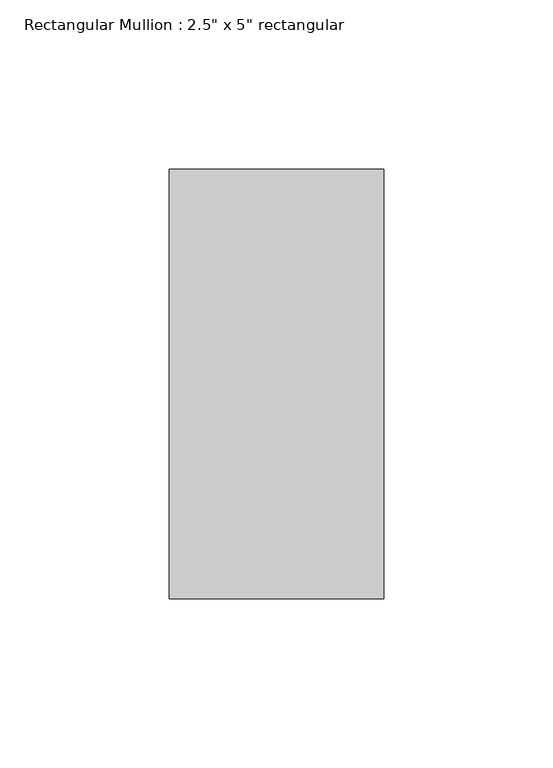
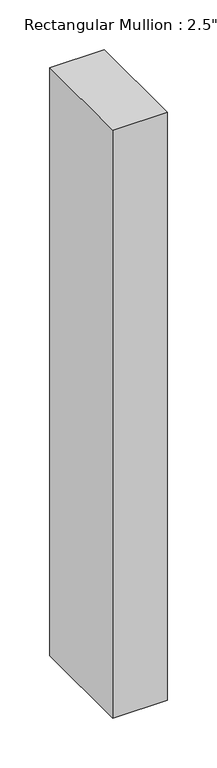
"""IFC4 building model written with IfcOpenShell, lengths in millimetres: member geometry."""

from ifc_helpers import new_model, si_unit, frame, origin, place, context, project, spatial, polyline, outline, extrude, source, transform, mapped, element, save


def member_695b83e4(model_context):
    return source(origin(), model_context, "Body", "SweptSolid", [
        extrude(outline(polyline([(0.0, 63.5), (0.0, -63.5), (-63.5, -63.5), (-63.5, 63.5), (0.0, 63.5)])), frame((0.0, 0.0, -724.0034475), z_axis=(0.0, 0.0, 1.0), x_axis=(1.0, 0.0, 0.0)), (0.0, 0.0, 1.0), 724.0034475),
    ])


if __name__ == "__main__":
    model = new_model("IFC4")
    model_context = context("Model", 3, world=origin())
    ifc_project = project(units=[si_unit("LENGTHUNIT", "METRE", prefix="MILLI")], contexts=[model_context])
    site = spatial("IfcSite", under=ifc_project)
    building = spatial("IfcBuilding", under=site)
    placement = place(None, origin())
    member_shape = member_695b83e4(model_context)
    element("IfcMember", 1, ObjectType="Rectangular Mullion : 2.5\" x 5\" rectangular", at=placement, inside=building, context=model_context, shape_type="MappedRepresentation", body=[
        mapped(member_shape, transform((0.0, 0.0, 0.0), x_axis=(1.0, 0.0, 0.0), y_axis=(0.0, 1.0, 0.0), z_axis=(0.0, 0.0, 1.0))),
    ])
    save(model, "model.ifc")

# Revit data of these elements
# Type "Rectangular Mullion : 2.5\" x 5\" rectangular"
#   built-in parameter 1007304 = 0.416667 (stored number, unit not read)
#   built-in parameter 1007301 = 0.104167 (stored number, unit not read)
#   built-in parameter 1007300 = 0.104167 (stored number, unit not read)
# Element 1 (IfcMember, "Rectangular Mullion : 2.5\" x 5\" rectangular")
#   Materials on its faces: "Aluminum"
# Materials
#   "Aluminum": class "Metal", colour RGB 247 247 247, transparency 0, Description = "Aluminum 6061", Cost = 0
